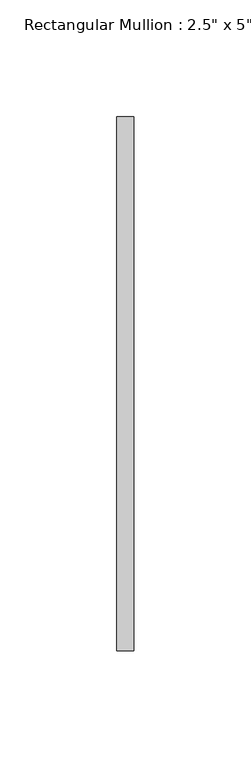
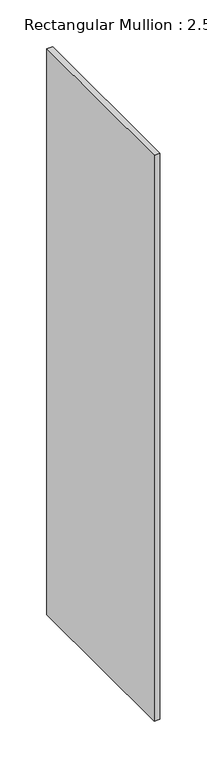
"""IFC4 building model written with IfcOpenShell, lengths in millimetres: member geometry."""

from ifc_helpers import new_model, si_unit, frame, origin, place, context, project, spatial, polyline, outline, extrude, source, transform, mapped, element, save


def member_3bd50dc0(model_context):
    return source(origin(), model_context, "Body", "SweptSolid", [
        extrude(outline(polyline([(3.6195, 114.3), (3.6195, -114.3), (-3.6195, -114.3), (-3.6195, 114.3), (3.6195, 114.3)])), frame((0.0, 0.0, -736.6), z_axis=(0.0, 0.0, 1.0), x_axis=(1.0, 0.0, 0.0)), (0.0, 0.0, 1.0), 736.6),
    ])


if __name__ == "__main__":
    model = new_model("IFC4")
    model_context = context("Model", 3, world=origin())
    ifc_project = project(units=[si_unit("LENGTHUNIT", "METRE", prefix="MILLI")], contexts=[model_context])
    site = spatial("IfcSite", under=ifc_project)
    building = spatial("IfcBuilding", under=site)
    placement = place(None, origin())
    member_shape = member_3bd50dc0(model_context)
    element("IfcMember", 1, ObjectType="Rectangular Mullion : 2.5\" x 5\" rectangular", at=placement, inside=building, context=model_context, shape_type="MappedRepresentation", body=[
        mapped(member_shape, transform((0.0, 0.0, 0.0), x_axis=(1.0, 0.0, 0.0), y_axis=(0.0, 1.0, 0.0), z_axis=(0.0, 0.0, 1.0))),
    ])
    save(model, "model.ifc")

# Revit data of these elements
# Type "Rectangular Mullion : 2.5\" x 5\" rectangular"
#   built-in parameter 1007304 = 0.75 (stored number, unit not read)
#   built-in parameter 1007301 = 0.011875 (stored number, unit not read)
#   built-in parameter 1007300 = 0.011875 (stored number, unit not read)
# Element 1 (IfcMember, "Rectangular Mullion : 2.5\" x 5\" rectangular")
#   Materials on its faces: "WINDOW GLASS MATERIAL"
# Materials
#   "WINDOW GLASS MATERIAL": class "Generic", colour RGB 120 120 120, transparency 0, Cost = 0
